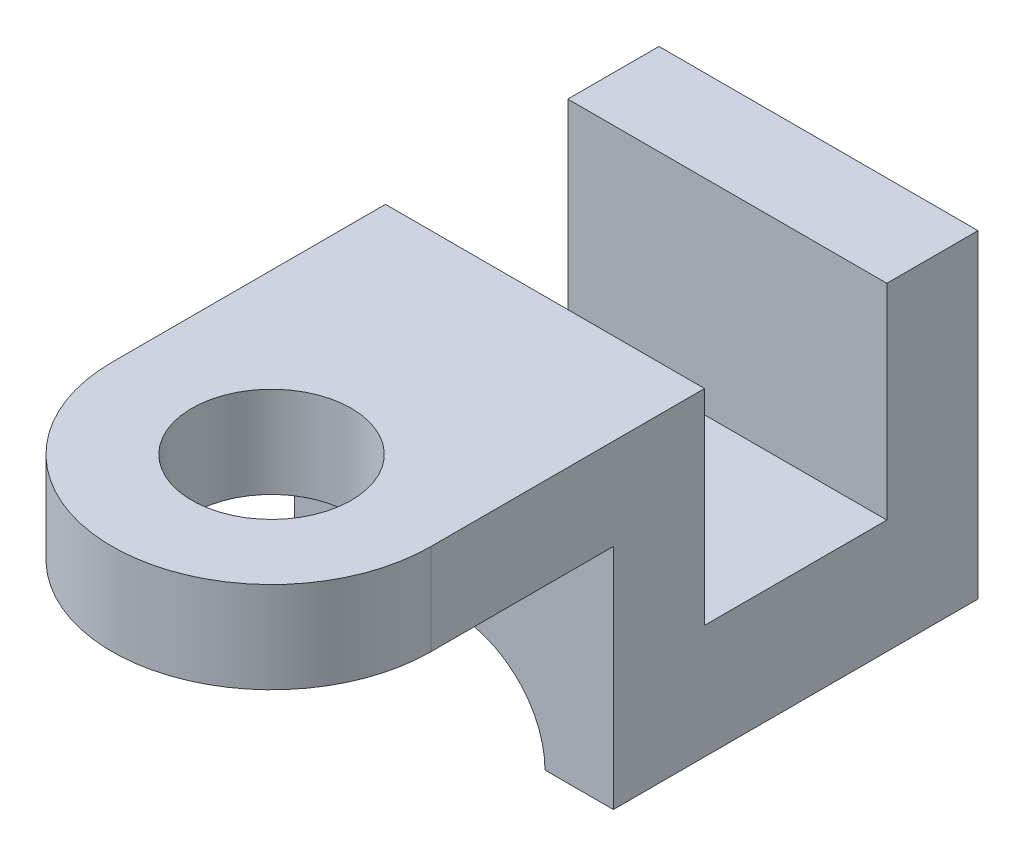
ISO-10303-21;
HEADER;
FILE_DESCRIPTION(('STEP AP214'),'2;1');
FILE_NAME('part.step','',(''),(''),'','','');
FILE_SCHEMA(('AUTOMOTIVE_DESIGN { 1 0 10303 214 1 1 1 1 }'));
ENDSEC;
DATA;
#1=APPLICATION_CONTEXT('core data for automotive mechanical design processes');
#2=APPLICATION_PROTOCOL_DEFINITION('international standard','automotive_design',2000,#1);
#3=PRODUCT_CONTEXT('',#1,'mechanical');
#4=PRODUCT('Part','Part','',(#3));
#5=PRODUCT_RELATED_PRODUCT_CATEGORY('part','',(#4));
#6=PRODUCT_DEFINITION_FORMATION('','',#4);
#7=PRODUCT_DEFINITION_CONTEXT('part definition',#1,'design');
#8=PRODUCT_DEFINITION('design','',#6,#7);
#9=PRODUCT_DEFINITION_SHAPE('','',#8);
#10=(LENGTH_UNIT() NAMED_UNIT(*) SI_UNIT(.MILLI.,.METRE.));
#11=(NAMED_UNIT(*) PLANE_ANGLE_UNIT() SI_UNIT($,.RADIAN.));
#12=(NAMED_UNIT(*) SI_UNIT($,.STERADIAN.) SOLID_ANGLE_UNIT());
#13=UNCERTAINTY_MEASURE_WITH_UNIT(LENGTH_MEASURE(1.E-05),#10,'distance_accuracy_value','');
#14=(GEOMETRIC_REPRESENTATION_CONTEXT(3) GLOBAL_UNCERTAINTY_ASSIGNED_CONTEXT((#13)) GLOBAL_UNIT_ASSIGNED_CONTEXT((#10,
#11,#12)) REPRESENTATION_CONTEXT('',''));
#15=CARTESIAN_POINT('',(0.,0.,0.));
#16=DIRECTION('',(0.,0.,1.));
#17=DIRECTION('',(1.,0.,0.));
#18=AXIS2_PLACEMENT_3D('',#15,#16,#17);
#19=CARTESIAN_POINT('',(70.,-45.,80.));
#20=DIRECTION('',(0.,0.,1.));
#21=DIRECTION('',(1.,0.,0.));
#22=AXIS2_PLACEMENT_3D('',#19,#20,#21);
#23=PLANE('',#22);
#24=DIRECTION('',(0.,1.,0.));
#25=VECTOR('',#24,1.);
#26=CARTESIAN_POINT('',(70.,-45.,80.));
#27=LINE('',#26,#25);
#28=CARTESIAN_POINT('',(70.,-70.,80.));
#29=VERTEX_POINT('',#28);
#30=CARTESIAN_POINT('',(70.,-20.,80.));
#31=VERTEX_POINT('',#30);
#32=EDGE_CURVE('E188',#29,#31,#27,.T.);
#33=ORIENTED_EDGE('',*,*,#32,.T.);
#34=DIRECTION('',(-1.,0.,0.));
#35=VECTOR('',#34,1.);
#36=CARTESIAN_POINT('',(0.,-20.,80.));
#37=LINE('',#36,#35);
#38=CARTESIAN_POINT('',(0.,-20.,80.));
#39=VERTEX_POINT('',#38);
#40=EDGE_CURVE('E147',#31,#39,#37,.T.);
#41=ORIENTED_EDGE('',*,*,#40,.T.);
#42=DIRECTION('',(0.,1.,0.));
#43=VECTOR('',#42,1.);
#44=CARTESIAN_POINT('',(0.,-45.,80.));
#45=LINE('',#44,#43);
#46=CARTESIAN_POINT('',(0.,-70.,80.));
#47=VERTEX_POINT('',#46);
#48=EDGE_CURVE('E158',#47,#39,#45,.T.);
#49=ORIENTED_EDGE('',*,*,#48,.F.);
#50=DIRECTION('',(-1.,0.,0.));
#51=VECTOR('',#50,1.);
#52=CARTESIAN_POINT('',(70.,-70.,80.));
#53=LINE('',#52,#51);
#54=CARTESIAN_POINT('',(15.,-70.,80.));
#55=VERTEX_POINT('',#54);
#56=EDGE_CURVE('E194',#55,#47,#53,.T.);
#57=ORIENTED_EDGE('',*,*,#56,.F.);
#58=CARTESIAN_POINT('',(35.,-70.,80.));
#59=DIRECTION('',(0.,0.,1.));
#60=DIRECTION('',(1.,0.,0.));
#61=AXIS2_PLACEMENT_3D('',#58,#59,#60);
#62=CIRCLE('',#61,20.);
#63=CARTESIAN_POINT('',(55.,-70.,80.));
#64=VERTEX_POINT('',#63);
#65=EDGE_CURVE('E168',#64,#55,#62,.T.);
#66=ORIENTED_EDGE('',*,*,#65,.F.);
#67=EDGE_CURVE('E193',#29,#64,#53,.T.);
#68=ORIENTED_EDGE('',*,*,#67,.F.);
#69=EDGE_LOOP('',(#33,#41,#49,#57,#66,#68));
#70=FACE_BOUND('',#69,.T.);
#71=ADVANCED_FACE('F44',(#70),#23,.T.);
#72=CARTESIAN_POINT('',(70.,-70.,20.));
#73=DIRECTION('',(0.,1.,0.));
#74=DIRECTION('',(0.,0.,1.));
#75=AXIS2_PLACEMENT_3D('',#72,#73,#74);
#76=PLANE('',#75);
#77=DIRECTION('',(1.,0.,0.));
#78=VECTOR('',#77,1.);
#79=CARTESIAN_POINT('',(70.,-70.,0.));
#80=LINE('',#79,#78);
#81=CARTESIAN_POINT('',(0.,-70.,0.));
#82=VERTEX_POINT('',#81);
#83=CARTESIAN_POINT('',(15.,-70.,0.));
#84=VERTEX_POINT('',#83);
#85=EDGE_CURVE('E219',#82,#84,#80,.T.);
#86=ORIENTED_EDGE('',*,*,#85,.T.);
#87=DIRECTION('',(0.,0.,1.));
#88=VECTOR('',#87,1.);
#89=CARTESIAN_POINT('',(15.,-70.,0.));
#90=LINE('',#89,#88);
#91=EDGE_CURVE('E171',#84,#55,#90,.T.);
#92=ORIENTED_EDGE('',*,*,#91,.T.);
#93=ORIENTED_EDGE('',*,*,#56,.T.);
#94=DIRECTION('',(0.,0.,-1.));
#95=VECTOR('',#94,1.);
#96=CARTESIAN_POINT('',(0.,-70.,20.));
#97=LINE('',#96,#95);
#98=EDGE_CURVE('E11',#47,#82,#97,.T.);
#99=ORIENTED_EDGE('',*,*,#98,.T.);
#100=EDGE_LOOP('',(#86,#92,#93,#99));
#101=FACE_BOUND('',#100,.T.);
#102=ADVANCED_FACE('F261',(#101),#76,.F.);
#103=CARTESIAN_POINT('',(0.,-70.,20.));
#104=DIRECTION('',(1.,0.,0.));
#105=DIRECTION('',(0.,0.,-1.));
#106=AXIS2_PLACEMENT_3D('',#103,#104,#105);
#107=PLANE('',#106);
#108=DIRECTION('',(0.,-1.,0.));
#109=VECTOR('',#108,1.);
#110=CARTESIAN_POINT('',(0.,-70.,0.));
#111=LINE('',#110,#109);
#112=CARTESIAN_POINT('',(0.,0.,0.));
#113=VERTEX_POINT('',#112);
#114=EDGE_CURVE('E207',#113,#82,#111,.T.);
#115=ORIENTED_EDGE('',*,*,#114,.T.);
#116=ORIENTED_EDGE('',*,*,#98,.F.);
#117=ORIENTED_EDGE('',*,*,#48,.T.);
#118=DIRECTION('',(0.,0.,1.));
#119=VECTOR('',#118,1.);
#120=CARTESIAN_POINT('',(0.,-20.,80.));
#121=LINE('',#120,#119);
#122=CARTESIAN_POINT('',(0.,-20.,120.));
#123=VERTEX_POINT('',#122);
#124=EDGE_CURVE('E58',#39,#123,#121,.T.);
#125=ORIENTED_EDGE('',*,*,#124,.T.);
#126=DIRECTION('',(0.,1.,0.));
#127=VECTOR('',#126,1.);
#128=CARTESIAN_POINT('',(0.,-20.,120.));
#129=LINE('',#128,#127);
#130=CARTESIAN_POINT('',(0.,0.,120.));
#131=VERTEX_POINT('',#130);
#132=EDGE_CURVE('E140',#123,#131,#129,.T.);
#133=ORIENTED_EDGE('',*,*,#132,.T.);
#134=DIRECTION('',(0.,0.,-1.));
#135=VECTOR('',#134,1.);
#136=CARTESIAN_POINT('',(0.,0.,80.));
#137=LINE('',#136,#135);
#138=CARTESIAN_POINT('',(0.,0.,60.));
#139=VERTEX_POINT('',#138);
#140=EDGE_CURVE('E184',#131,#139,#137,.T.);
#141=ORIENTED_EDGE('',*,*,#140,.T.);
#142=DIRECTION('',(0.,-1.,0.));
#143=VECTOR('',#142,1.);
#144=CARTESIAN_POINT('',(0.,-45.,60.));
#145=LINE('',#144,#143);
#146=CARTESIAN_POINT('',(0.,-45.,60.));
#147=VERTEX_POINT('',#146);
#148=EDGE_CURVE('E182',#139,#147,#145,.T.);
#149=ORIENTED_EDGE('',*,*,#148,.T.);
#150=DIRECTION('',(0.,0.,-1.));
#151=VECTOR('',#150,1.);
#152=CARTESIAN_POINT('',(0.,-45.,20.));
#153=LINE('',#152,#151);
#154=CARTESIAN_POINT('',(0.,-45.,20.));
#155=VERTEX_POINT('',#154);
#156=EDGE_CURVE('E204',#147,#155,#153,.T.);
#157=ORIENTED_EDGE('',*,*,#156,.T.);
#158=DIRECTION('',(0.,-1.,0.));
#159=VECTOR('',#158,1.);
#160=CARTESIAN_POINT('',(0.,-70.,20.));
#161=LINE('',#160,#159);
#162=CARTESIAN_POINT('',(0.,0.,20.));
#163=VERTEX_POINT('',#162);
#164=EDGE_CURVE('E210',#163,#155,#161,.T.);
#165=ORIENTED_EDGE('',*,*,#164,.F.);
#166=DIRECTION('',(0.,0.,-1.));
#167=VECTOR('',#166,1.);
#168=CARTESIAN_POINT('',(0.,0.,20.));
#169=LINE('',#168,#167);
#170=EDGE_CURVE('E213',#163,#113,#169,.T.);
#171=ORIENTED_EDGE('',*,*,#170,.T.);
#172=EDGE_LOOP('',(#115,#116,#117,#125,#133,#141,#149,#157,#165,#171));
#173=FACE_BOUND('',#172,.T.);
#174=ADVANCED_FACE('F50',(#173),#107,.F.);
#175=ORIENTED_EDGE('',*,*,#67,.T.);
#176=DIRECTION('',(0.,0.,1.));
#177=VECTOR('',#176,1.);
#178=CARTESIAN_POINT('',(55.,-70.,0.));
#179=LINE('',#178,#177);
#180=CARTESIAN_POINT('',(55.,-70.,0.));
#181=VERTEX_POINT('',#180);
#182=EDGE_CURVE('E69',#181,#64,#179,.T.);
#183=ORIENTED_EDGE('',*,*,#182,.F.);
#184=CARTESIAN_POINT('',(70.,-70.,0.));
#185=VERTEX_POINT('',#184);
#186=EDGE_CURVE('E220',#181,#185,#80,.T.);
#187=ORIENTED_EDGE('',*,*,#186,.T.);
#188=DIRECTION('',(0.,0.,-1.));
#189=VECTOR('',#188,1.);
#190=CARTESIAN_POINT('',(70.,-70.,20.));
#191=LINE('',#190,#189);
#192=EDGE_CURVE('E52',#29,#185,#191,.T.);
#193=ORIENTED_EDGE('',*,*,#192,.F.);
#194=EDGE_LOOP('',(#175,#183,#187,#193));
#195=FACE_BOUND('',#194,.T.);
#196=ADVANCED_FACE('F265',(#195),#76,.F.);
#197=CARTESIAN_POINT('',(70.,0.,20.));
#198=DIRECTION('',(-1.,0.,0.));
#199=DIRECTION('',(0.,0.,1.));
#200=AXIS2_PLACEMENT_3D('',#197,#198,#199);
#201=PLANE('',#200);
#202=DIRECTION('',(0.,1.,0.));
#203=VECTOR('',#202,1.);
#204=CARTESIAN_POINT('',(70.,0.,0.));
#205=LINE('',#204,#203);
#206=CARTESIAN_POINT('',(70.,0.,0.));
#207=VERTEX_POINT('',#206);
#208=EDGE_CURVE('E223',#185,#207,#205,.T.);
#209=ORIENTED_EDGE('',*,*,#208,.T.);
#210=DIRECTION('',(0.,0.,-1.));
#211=VECTOR('',#210,1.);
#212=CARTESIAN_POINT('',(70.,0.,20.));
#213=LINE('',#212,#211);
#214=CARTESIAN_POINT('',(70.,0.,20.));
#215=VERTEX_POINT('',#214);
#216=EDGE_CURVE('E228',#215,#207,#213,.T.);
#217=ORIENTED_EDGE('',*,*,#216,.F.);
#218=DIRECTION('',(0.,1.,0.));
#219=VECTOR('',#218,1.);
#220=CARTESIAN_POINT('',(70.,0.,20.));
#221=LINE('',#220,#219);
#222=CARTESIAN_POINT('',(70.,-45.,20.));
#223=VERTEX_POINT('',#222);
#224=EDGE_CURVE('E208',#223,#215,#221,.T.);
#225=ORIENTED_EDGE('',*,*,#224,.F.);
#226=DIRECTION('',(0.,0.,1.));
#227=VECTOR('',#226,1.);
#228=CARTESIAN_POINT('',(70.,-45.,60.));
#229=LINE('',#228,#227);
#230=CARTESIAN_POINT('',(70.,-45.,60.));
#231=VERTEX_POINT('',#230);
#232=EDGE_CURVE('E203',#223,#231,#229,.T.);
#233=ORIENTED_EDGE('',*,*,#232,.T.);
#234=DIRECTION('',(0.,1.,0.));
#235=VECTOR('',#234,1.);
#236=CARTESIAN_POINT('',(70.,0.,60.));
#237=LINE('',#236,#235);
#238=CARTESIAN_POINT('',(70.,0.,60.));
#239=VERTEX_POINT('',#238);
#240=EDGE_CURVE('E177',#231,#239,#237,.T.);
#241=ORIENTED_EDGE('',*,*,#240,.T.);
#242=DIRECTION('',(0.,0.,-1.));
#243=VECTOR('',#242,1.);
#244=CARTESIAN_POINT('',(70.,0.,80.));
#245=LINE('',#244,#243);
#246=CARTESIAN_POINT('',(70.,0.,120.));
#247=VERTEX_POINT('',#246);
#248=EDGE_CURVE('E190',#247,#239,#245,.T.);
#249=ORIENTED_EDGE('',*,*,#248,.F.);
#250=DIRECTION('',(0.,1.,0.));
#251=VECTOR('',#250,1.);
#252=CARTESIAN_POINT('',(70.,-20.,120.));
#253=LINE('',#252,#251);
#254=CARTESIAN_POINT('',(70.,-20.,120.));
#255=VERTEX_POINT('',#254);
#256=EDGE_CURVE('E143',#255,#247,#253,.T.);
#257=ORIENTED_EDGE('',*,*,#256,.F.);
#258=DIRECTION('',(0.,0.,-1.));
#259=VECTOR('',#258,1.);
#260=CARTESIAN_POINT('',(70.,-20.,80.));
#261=LINE('',#260,#259);
#262=EDGE_CURVE('E148',#255,#31,#261,.T.);
#263=ORIENTED_EDGE('',*,*,#262,.T.);
#264=ORIENTED_EDGE('',*,*,#32,.F.);
#265=ORIENTED_EDGE('',*,*,#192,.T.);
#266=EDGE_LOOP('',(#209,#217,#225,#233,#241,#249,#257,#263,#264,#265));
#267=FACE_BOUND('',#266,.T.);
#268=ADVANCED_FACE('F235',(#267),#201,.F.);
#269=CARTESIAN_POINT('',(0.,0.,20.));
#270=DIRECTION('',(0.,-1.,0.));
#271=DIRECTION('',(0.,0.,-1.));
#272=AXIS2_PLACEMENT_3D('',#269,#270,#271);
#273=PLANE('',#272);
#274=DIRECTION('',(-1.,0.,0.));
#275=VECTOR('',#274,1.);
#276=CARTESIAN_POINT('',(0.,0.,0.));
#277=LINE('',#276,#275);
#278=EDGE_CURVE('E212',#207,#113,#277,.T.);
#279=ORIENTED_EDGE('',*,*,#278,.T.);
#280=ORIENTED_EDGE('',*,*,#170,.F.);
#281=DIRECTION('',(-1.,0.,0.));
#282=VECTOR('',#281,1.);
#283=CARTESIAN_POINT('',(0.,0.,20.));
#284=LINE('',#283,#282);
#285=EDGE_CURVE('E214',#215,#163,#284,.T.);
#286=ORIENTED_EDGE('',*,*,#285,.F.);
#287=ORIENTED_EDGE('',*,*,#216,.T.);
#288=EDGE_LOOP('',(#279,#280,#286,#287));
#289=FACE_BOUND('',#288,.T.);
#290=ADVANCED_FACE('F243',(#289),#273,.F.);
#291=CARTESIAN_POINT('',(0.,0.,20.));
#292=DIRECTION('',(0.,0.,-1.));
#293=DIRECTION('',(-1.,0.,0.));
#294=AXIS2_PLACEMENT_3D('',#291,#292,#293);
#295=PLANE('',#294);
#296=ORIENTED_EDGE('',*,*,#164,.T.);
#297=DIRECTION('',(1.,0.,0.));
#298=VECTOR('',#297,1.);
#299=CARTESIAN_POINT('',(70.,-45.,20.));
#300=LINE('',#299,#298);
#301=EDGE_CURVE('E199',#155,#223,#300,.T.);
#302=ORIENTED_EDGE('',*,*,#301,.T.);
#303=ORIENTED_EDGE('',*,*,#224,.T.);
#304=ORIENTED_EDGE('',*,*,#285,.T.);
#305=EDGE_LOOP('',(#296,#302,#303,#304));
#306=FACE_BOUND('',#305,.T.);
#307=ADVANCED_FACE('F248',(#306),#295,.F.);
#308=CARTESIAN_POINT('',(0.,0.,0.));
#309=DIRECTION('',(0.,0.,-1.));
#310=DIRECTION('',(-1.,0.,0.));
#311=AXIS2_PLACEMENT_3D('',#308,#309,#310);
#312=PLANE('',#311);
#313=CARTESIAN_POINT('',(35.,-70.,0.));
#314=DIRECTION('',(0.,0.,1.));
#315=DIRECTION('',(1.,0.,0.));
#316=AXIS2_PLACEMENT_3D('',#313,#314,#315);
#317=CIRCLE('',#316,20.);
#318=EDGE_CURVE('E166',#181,#84,#317,.T.);
#319=ORIENTED_EDGE('',*,*,#318,.T.);
#320=ORIENTED_EDGE('',*,*,#85,.F.);
#321=ORIENTED_EDGE('',*,*,#114,.F.);
#322=ORIENTED_EDGE('',*,*,#278,.F.);
#323=ORIENTED_EDGE('',*,*,#208,.F.);
#324=ORIENTED_EDGE('',*,*,#186,.F.);
#325=EDGE_LOOP('',(#319,#320,#321,#322,#323,#324));
#326=FACE_BOUND('',#325,.T.);
#327=ADVANCED_FACE('F237',(#326),#312,.T.);
#328=CARTESIAN_POINT('',(0.,-45.,0.));
#329=DIRECTION('',(0.,1.,0.));
#330=DIRECTION('',(0.,0.,1.));
#331=AXIS2_PLACEMENT_3D('',#328,#329,#330);
#332=PLANE('',#331);
#333=DIRECTION('',(1.,0.,0.));
#334=VECTOR('',#333,1.);
#335=CARTESIAN_POINT('',(70.,-45.,60.));
#336=LINE('',#335,#334);
#337=EDGE_CURVE('E172',#147,#231,#336,.T.);
#338=ORIENTED_EDGE('',*,*,#337,.T.);
#339=ORIENTED_EDGE('',*,*,#232,.F.);
#340=ORIENTED_EDGE('',*,*,#301,.F.);
#341=ORIENTED_EDGE('',*,*,#156,.F.);
#342=EDGE_LOOP('',(#338,#339,#340,#341));
#343=FACE_BOUND('',#342,.T.);
#344=ADVANCED_FACE('F255',(#343),#332,.T.);
#345=CARTESIAN_POINT('',(0.,0.,80.));
#346=DIRECTION('',(0.,-1.,0.));
#347=DIRECTION('',(0.,0.,-1.));
#348=AXIS2_PLACEMENT_3D('',#345,#346,#347);
#349=PLANE('',#348);
#350=CARTESIAN_POINT('',(35.,0.,120.));
#351=DIRECTION('',(0.,-1.,0.));
#352=DIRECTION('',(0.,0.,-1.));
#353=AXIS2_PLACEMENT_3D('',#350,#351,#352);
#354=CIRCLE('',#353,17.5);
#355=CARTESIAN_POINT('',(35.,0.,102.5));
#356=VERTEX_POINT('',#355);
#357=EDGE_CURVE('E156',#356,#356,#354,.T.);
#358=ORIENTED_EDGE('',*,*,#357,.T.);
#359=EDGE_LOOP('',(#358));
#360=FACE_BOUND('',#359,.T.);
#361=DIRECTION('',(-1.,0.,0.));
#362=VECTOR('',#361,1.);
#363=CARTESIAN_POINT('',(0.,0.,60.));
#364=LINE('',#363,#362);
#365=EDGE_CURVE('E181',#239,#139,#364,.T.);
#366=ORIENTED_EDGE('',*,*,#365,.T.);
#367=ORIENTED_EDGE('',*,*,#140,.F.);
#368=CARTESIAN_POINT('',(35.,0.,120.));
#369=DIRECTION('',(0.,1.,0.));
#370=DIRECTION('',(0.,0.,1.));
#371=AXIS2_PLACEMENT_3D('',#368,#369,#370);
#372=CIRCLE('',#371,35.);
#373=EDGE_CURVE('E145',#131,#247,#372,.T.);
#374=ORIENTED_EDGE('',*,*,#373,.T.);
#375=ORIENTED_EDGE('',*,*,#248,.T.);
#376=EDGE_LOOP('',(#366,#367,#374,#375));
#377=FACE_BOUND('',#376,.T.);
#378=ADVANCED_FACE('F256',(#360,#377),#349,.F.);
#379=CARTESIAN_POINT('',(0.,0.,60.));
#380=DIRECTION('',(0.,0.,-1.));
#381=DIRECTION('',(-1.,0.,0.));
#382=AXIS2_PLACEMENT_3D('',#379,#380,#381);
#383=PLANE('',#382);
#384=ORIENTED_EDGE('',*,*,#337,.F.);
#385=ORIENTED_EDGE('',*,*,#148,.F.);
#386=ORIENTED_EDGE('',*,*,#365,.F.);
#387=ORIENTED_EDGE('',*,*,#240,.F.);
#388=EDGE_LOOP('',(#384,#385,#386,#387));
#389=FACE_BOUND('',#388,.T.);
#390=ADVANCED_FACE('F257',(#389),#383,.T.);
#391=CARTESIAN_POINT('',(35.,-70.,0.));
#392=DIRECTION('',(0.,0.,1.));
#393=DIRECTION('',(1.,0.,0.));
#394=AXIS2_PLACEMENT_3D('',#391,#392,#393);
#395=CYLINDRICAL_SURFACE('',#394,20.);
#396=ORIENTED_EDGE('',*,*,#65,.T.);
#397=ORIENTED_EDGE('',*,*,#91,.F.);
#398=ORIENTED_EDGE('',*,*,#318,.F.);
#399=ORIENTED_EDGE('',*,*,#182,.T.);
#400=EDGE_LOOP('',(#396,#397,#398,#399));
#401=FACE_BOUND('',#400,.T.);
#402=ADVANCED_FACE('F307',(#401),#395,.F.);
#403=CARTESIAN_POINT('',(35.,-20.,120.));
#404=DIRECTION('',(0.,1.,0.));
#405=DIRECTION('',(0.,0.,1.));
#406=AXIS2_PLACEMENT_3D('',#403,#404,#405);
#407=CYLINDRICAL_SURFACE('',#406,35.);
#408=ORIENTED_EDGE('',*,*,#373,.F.);
#409=ORIENTED_EDGE('',*,*,#132,.F.);
#410=CARTESIAN_POINT('',(35.,-20.,120.));
#411=DIRECTION('',(0.,1.,0.));
#412=DIRECTION('',(0.,0.,1.));
#413=AXIS2_PLACEMENT_3D('',#410,#411,#412);
#414=CIRCLE('',#413,35.);
#415=EDGE_CURVE('E137',#123,#255,#414,.T.);
#416=ORIENTED_EDGE('',*,*,#415,.T.);
#417=ORIENTED_EDGE('',*,*,#256,.T.);
#418=EDGE_LOOP('',(#408,#409,#416,#417));
#419=FACE_BOUND('',#418,.T.);
#420=ADVANCED_FACE('F136',(#419),#407,.T.);
#421=CARTESIAN_POINT('',(35.,-20.,120.));
#422=DIRECTION('',(0.,1.,0.));
#423=DIRECTION('',(0.,0.,1.));
#424=AXIS2_PLACEMENT_3D('',#421,#422,#423);
#425=PLANE('',#424);
#426=CARTESIAN_POINT('',(35.,-20.,120.));
#427=DIRECTION('',(0.,-1.,0.));
#428=DIRECTION('',(0.,0.,-1.));
#429=AXIS2_PLACEMENT_3D('',#426,#427,#428);
#430=CIRCLE('',#429,17.5);
#431=CARTESIAN_POINT('',(35.,-20.,102.5));
#432=VERTEX_POINT('',#431);
#433=EDGE_CURVE('E163',#432,#432,#430,.T.);
#434=ORIENTED_EDGE('',*,*,#433,.F.);
#435=EDGE_LOOP('',(#434));
#436=FACE_BOUND('',#435,.T.);
#437=ORIENTED_EDGE('',*,*,#124,.F.);
#438=ORIENTED_EDGE('',*,*,#40,.F.);
#439=ORIENTED_EDGE('',*,*,#262,.F.);
#440=ORIENTED_EDGE('',*,*,#415,.F.);
#441=EDGE_LOOP('',(#437,#438,#439,#440));
#442=FACE_BOUND('',#441,.T.);
#443=ADVANCED_FACE('F146',(#436,#442),#425,.F.);
#444=CARTESIAN_POINT('',(35.,0.,120.));
#445=DIRECTION('',(0.,-1.,0.));
#446=DIRECTION('',(0.,0.,-1.));
#447=AXIS2_PLACEMENT_3D('',#444,#445,#446);
#448=CYLINDRICAL_SURFACE('',#447,17.5);
#449=ORIENTED_EDGE('',*,*,#357,.F.);
#450=EDGE_LOOP('',(#449));
#451=FACE_BOUND('',#450,.T.);
#452=ORIENTED_EDGE('',*,*,#433,.T.);
#453=EDGE_LOOP('',(#452));
#454=FACE_BOUND('',#453,.T.);
#455=ADVANCED_FACE('F347',(#451,#454),#448,.F.);
#456=CLOSED_SHELL('',(#71,#102,#174,#196,#268,#290,#307,#327,#344,#378,#390,#402,#420,#443,#455));
#457=MANIFOLD_SOLID_BREP('B2',#456);
#458=ADVANCED_BREP_SHAPE_REPRESENTATION('',(#18,#457),#14);
#459=SHAPE_DEFINITION_REPRESENTATION(#9,#458);
ENDSEC;
END-ISO-10303-21;
